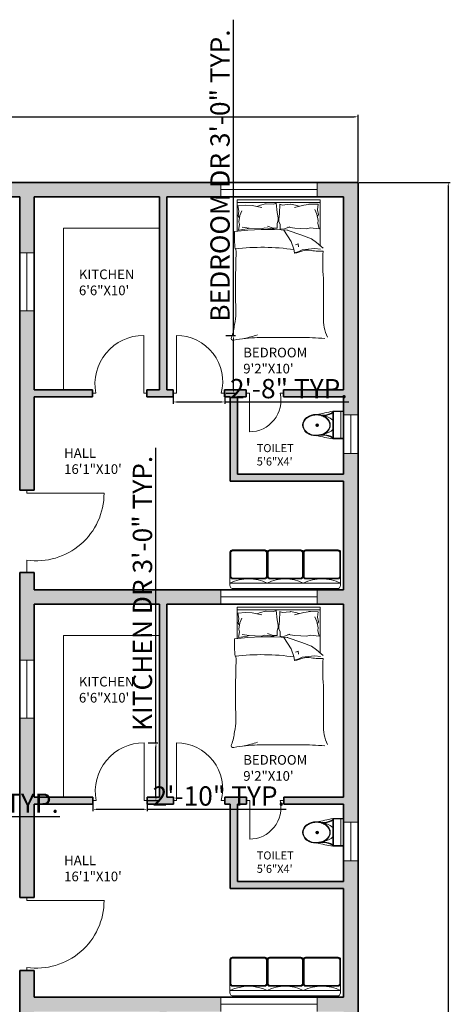
# Model space of a CAD drawing. Units: inches. Extents: x 1266 to 2869, y -408 to 3241.
# Tile 5 of 11: x 1748 to 2016, y 1767 to 2380. Entities that reach past the tile are written whole.
import ezdxf

# ---------------------------------------------------------------- set-up
doc = ezdxf.new("R2010")
doc.units = ezdxf.units.IN
for name, color, linetype, lineweight in [('A-ANNO-DIMS', 2, 'Continuous', 18), ('A-AREA-IDEN', 7, 'Continuous', 18), ('A-DOOR', 4, 'Continuous', 18), ('A-FLOR-CASE', 9, 'Continuous', 18), ('A-FLOR-FIXT', 9, 'Continuous', 18), ('A-FURN', 8, 'Continuous', 18), ('A-GLAZ', 4, 'Continuous', 18), ('A-WALL', 7, 'Continuous', 35), ('A-WALL-PATT', 251, 'Continuous', 13)]:
    doc.layers.add(name, color=color, linetype=linetype, lineweight=lineweight)
doc.styles.get("Standard").update_dxf_attribs({"font": 'arial.ttf'})
doc.dimstyles.new('ISO-25', dxfattribs={"dimtxt": 12, "dimasz": 2.5, "dimexe": 1.25, "dimexo": 0.625, "dimtad": 1, "dimdec": 0, "dimlunit": 3, "dimtxsty": 'Standard', "dimcen": 2.5, "dimadec": 0, "dimazin": 0, "dimtfac": 1, "dimtdec": 0, "dimtmove": 0, "dimatfit": 3, "dimfxl": 1, "dimarcsym": 0})

# ---------------------------------------------------------------- blocks, each defined once
blk = doc.blocks.new('A$C31115884')
for p, q in [((283, 498), (223, 498)), ((258, 466), (258, 523)), ((0, 200), (0, 0)), ((520, 200), (0, 200)), ((10, 190), (10, 10)), ((510, 190), (10, 190)), ((510, 10), (510, 190)), ((520, 0), (520, 200)), ((510, 54), (0, 54)), ((10, 10), (510, 10)), ((0, 0), (520, 0))]:
    blk.add_line(p, q)
blk.add_circle((256, 496), 23.6)
for centre, radius, start, end in [((2778, -205), 2807, 165.4549, 171.7133), ((-295, 403), 365, 324.2091, 9.3499), ((-295, 403), 375, 324.2091, 9.3499), ((139, 406), 293, 315.8436, 2.6563), ((806, 403), 375, 179.2036, 215.7909), ((806, 403), 365, 170.6501, 215.7909), ((3237, 905), 2807, 188.2867, 194.5451), ((384, 406), 293, 190.2774, 224.1564)]:
    blk.add_arc(centre, radius, start, end)
blk.add_ellipse((256, 510), major_axis=(0, -261), ratio=0.772727)
blk.add_open_spline([(256, 259), (263, 259), (270, 260), (288, 262), (299, 265), (320, 273), (330, 278), (350, 291), (360, 299), (378, 316), (386, 326), (402, 347), (409, 358), (421, 383), (427, 395), (436, 422), (440, 436), (445, 465), (447, 480), (448, 509), (448, 524), (445, 553), (443, 568), (436, 596), (432, 610), (422, 636), (416, 649), (402, 672), (395, 683), (379, 703), (370, 712), (351, 728), (341, 735), (321, 746), (310, 751), (289, 757), (278, 759), (256, 761), (245, 761), (223, 757), (212, 754), (191, 746), (181, 741), (161, 728), (151, 720), (133, 703), (125, 693), (110, 672), (103, 660), (90, 636), (85, 623), (76, 596), (72, 582), (67, 553), (66, 538), (64, 509), (65, 494), (68, 465), (70, 450), (77, 422), (81, 408), (91, 382), (97, 370), (111, 346), (118, 335), (135, 316), (144, 307), (162, 291), (172, 284), (193, 273), (203, 269), (225, 262), (236, 260), (250, 259), (253, 259), (256, 259)], degree=3, knots=[0, 0, 0, 0, 0.110105, 0.110105, 0.285049, 0.285049, 0.459994, 0.459994, 0.634938, 0.634938, 0.809882, 0.809882, 0.984827, 0.984827, 1.159771, 1.159771, 1.334715, 1.334715, 1.50966, 1.50966, 1.684604, 1.684604, 1.859549, 1.859549, 2.034493, 2.034493, 2.209437, 2.209437, 2.384382, 2.384382, 2.559326, 2.559326, 2.73427, 2.73427, 2.909215, 2.909215, 3.084159, 3.084159, 3.259103, 3.259103, 3.434048, 3.434048, 3.608992, 3.608992, 3.783936, 3.783936, 3.958881, 3.958881, 4.133825, 4.133825, 4.30877, 4.30877, 4.483714, 4.483714, 4.658658, 4.658658, 4.833603, 4.833603, 5.008547, 5.008547, 5.183491, 5.183491, 5.358436, 5.358436, 5.53338, 5.53338, 5.708324, 5.708324, 5.883269, 5.883269, 6.058213, 6.058213, 6.233158, 6.233158, 6.283185, 6.283185, 6.283185, 6.283185])
blk = doc.blocks.new('*D2')
at = {"layer": 'A-ANNO-DIMS', "color": 0, "lineweight": -2, "transparency": 16777216}
for p, q in [((1475.69, 2278.97), (1475.69, 2320.42)), ((1478.19, 2319.17), (1956.19, 2319.17)), ((1958.69, 2278.97), (1958.69, 2320.42))]:
    blk.add_line(p, q, dxfattribs=at)
at = {"layer": 'A-ANNO-DIMS', "color": 0, "transparency": 16777216}
for points in [[(1478.19, 2319.59), (1478.19, 2318.76), (1475.69, 2319.17)], [(1956.19, 2319.59), (1956.19, 2318.76), (1958.69, 2319.17)]]:
    blk.add_solid(points, dxfattribs=at)
at = {"layer": 'Defpoints', "color": 0, "transparency": 16777216}
for p in [(1958.69, 2319.17), (1475.69, 2278.35), (1958.69, 2278.35)]:
    blk.add_point(p, dxfattribs=at)
at = {"layer": 'A-ANNO-DIMS', "color": 0, "transparency": 16777216, "insert": (1717.19, 2325.93), "char_height": 12, "attachment_point": 5}
blk.add_mtext('40\'-3"', dxfattribs=at)
blk = doc.blocks.new('*D3')
at = {"layer": 'A-ANNO-DIMS', "color": 0, "lineweight": -2, "transparency": 16777216}
for p, q in [((1959.32, 2278.35), (2016.1, 2278.35)), ((2014.85, 2275.85), (2014.85, 1179.85)), ((1959.32, 1177.35), (2016.1, 1177.35))]:
    blk.add_line(p, q, dxfattribs=at)
at = {"layer": 'A-ANNO-DIMS', "color": 0, "transparency": 16777216}
for points in [[(2014.43, 2275.85), (2015.27, 2275.85), (2014.85, 2278.35)], [(2014.43, 1179.85), (2015.27, 1179.85), (2014.85, 1177.35)]]:
    blk.add_solid(points, dxfattribs=at)
at = {"layer": 'Defpoints', "color": 0, "transparency": 16777216}
for p in [(1958.69, 2278.35), (1958.69, 1177.35), (2014.85, 1177.35)]:
    blk.add_point(p, dxfattribs=at)
at = {"layer": 'A-ANNO-DIMS', "color": 0, "transparency": 16777216, "insert": (2008.1, 1727.85), "char_height": 12, "attachment_point": 5, "rotation": 90}
blk.add_mtext('91\'-9"', dxfattribs=at)
blk = doc.blocks.new('BED-DOUBLE-2')
for p, q in [((3.76, 67.77), (3.76, 87.35)), ((3.76, 87.35), (55.42, 87.35)), ((55.42, 87.35), (55.42, 58.59)), ((3.76, 85.69), (55.42, 85.69)), ((4.21, 83.74), (8.84, 84.1)), ((4.21, 83.77), (4.84, 80.33)), ((4.84, 80.33), (4.37, 77.51)), ((5.46, 77.67), (6.55, 80.64)), ((8.84, 84.1), (8.96, 84.08)), ((8.96, 84.08), (13.09, 83.77)), ((13.09, 83.77), (19.03, 82.67)), ((16.06, 83.3), (18.25, 84.08)), ((18.25, 84.08), (21.37, 84.86)), ((21.37, 84.86), (21.72, 84.86)), ((21.72, 84.86), (26.53, 84.7)), ((26.53, 84.7), (28.09, 85.33)), ((28.09, 85.33), (28.71, 79.55)), ((30.24, 84.66), (29.98, 78.85)), ((31.84, 84.13), (30.24, 84.66)), ((36.63, 84.59), (31.84, 84.13)), ((36.98, 84.61), (36.63, 84.59)), ((40.14, 84.02), (36.98, 84.61)), ((45.31, 84.03), (39.45, 82.57)), ((42.38, 83.38), (40.14, 84.02)), ((49.42, 84.6), (45.31, 84.03)), ((54.17, 84.59), (48.33, 84.69)), ((48.33, 84.69), (49.42, 84.6)), ((53.31, 78.43), (52.03, 81.32)), ((54.17, 84.59), (53.76, 81.12)), ((53.76, 81.12), (54.41, 78.34)), ((4.37, 77.51), (4.99, 76.42)), ((4.84, 73.76), (5.46, 77.67)), ((5.15, 72.04), (4.84, 73.76)), ((28.71, 79.55), (29.34, 76.11)), ((29.34, 74.7), (28.71, 72.67)), ((29.34, 76.11), (29.34, 74.7)), ((29.98, 78.85), (29.57, 75.38)), ((29.57, 75.38), (29.66, 73.97)), ((29.66, 73.97), (30.41, 71.98)), ((54.17, 74.56), (53.31, 78.43)), ((54.41, 78.34), (53.85, 77.21)), ((53.97, 72.83), (54.17, 74.56)), ((4.52, 68.61), (5.15, 72.04)), ((10.03, 69.39), (4.52, 68.61)), ((6.9, 70.46), (11.26, 69.74)), ((11.26, 69.74), (10.03, 69.39)), ((11.26, 69.74), (18.84, 69.27)), ((18.84, 69.27), (20.95, 69.87)), ((20.95, 69.87), (26.5, 69.44)), ((26.06, 69.77), (22.66, 70.95)), ((28.71, 69.77), (26.06, 69.77)), ((28.71, 72.67), (28.71, 69.77)), ((30.41, 71.98), (30.59, 69.09)), ((30.59, 69.09), (33.24, 69.26)), ((32.71, 68.56), (37.24, 61.54)), ((33.24, 69.26), (36.56, 70.64)), ((43.94, 65.39), (34.92, 68.56)), ((35.2, 70.46), (39.56, 69.74)), ((39.56, 69.74), (47.14, 69.27)), ((47.14, 69.27), (49.26, 69.87)), ((49.26, 69.87), (54.81, 69.44)), ((54.81, 69.44), (53.97, 72.83)), ((37.24, 61.54), (39.08, 56.69)), ((49.96, 63.21), (43.94, 65.39)), ((53.15, 60.87), (49.96, 63.21)), ((39.08, 56.69), (39.42, 54.51)), ((39.42, 54.51), (42.1, 55.18)), ((40.12, 59.32), (41.78, 59.99)), ((41.87, 58.1), (41.78, 59.99, 4.18)), ((42.1, 55.18), (44.27, 56.19)), ((44.27, 56.19), (47.96, 56.69)), ((47.96, 56.69), (52.14, 57.02)), ((52.14, 57.02), (55.49, 56.69)), ((57.15, 57.36), (53.15, 60.87)), ((16.28, 1.69), (42.89, 1.69))]:
    blk.add_line(p, q)
for centre, radius, start, end in [((92.06, 65.63), 90.06, 178.72178, 185.60397), ((23.09, -109.45), 178.34, 86.08655, 96.78213), ((19.19, -81.63), 139.47, 81.78449, 96.90062), ((-180.86, 53.65), 183.89, 358.4762, 1.00819), ((33.68, 85.75), 32.06, 280.66171, 289.88058), ((47.29, 49.44), 6.73, 78.6608, 113.73842), ((55.49, 94.55), 39.11, 259.87628, 272.56571), ((197.03, 48.09), 139.99, 176.97912, 183.83645), ((39.61, 54.45), 0.199, 160.24637, 271.13765), ((524.11, 32.64), 521.39, 178.22771, 181.71854), ((-4874.07, 14.03), 4931.49, 0.00217, 0.28689), ((-29.08, 17.61), 32.04, 346.06484, 358.91125), ((82.33, 13.12), 24.93, 177.47136, 206.46809), ((-23.41, 11.38), 25.47, 337.97508, 356.652), ((1.18, 1.17), 1.18, 146.17358, 293.47814), ((23.16, -129.76), 131.62, 92.99578, 99.40907), ((-18.62, 112.98), 115.08, 283.38322, 287.70533), ((44.49, -142.12), 143.82, 84.4998, 90.63509)]:
    blk.add_arc(centre, radius, start, end)
blk = doc.blocks.new('SOFA-3-SEAT-2')
for points in [[(0, 22.36), (0, 7.74, 0.414214), (1.72, 6.02), (21.5, 6.02, 0.414214), (23.22, 7.74), (23.22, 22.36, 0.414214), (21.5, 24.08), (1.72, 24.08, 0.414214)], [(0.52, 22.36), (0.52, 7.74, 0.414214), (1.72, 6.53), (21.5, 6.53, 0.414214), (22.7, 7.74), (22.7, 22.36, 0.414214), (21.5, 23.56), (1.72, 23.56, 0.414214)], [(45.57, 22.36), (45.57, 7.74, -0.414214), (43.85, 6.02), (24.94, 6.02, -0.414214), (23.22, 7.74), (23.22, 22.36, -0.414214), (24.94, 24.08), (43.85, 24.08, -0.414214)], [(45.06, 22.36), (45.06, 7.74, -0.414214), (43.85, 6.53), (24.94, 6.53, -0.414214), (23.73, 7.74), (23.73, 22.36, -0.414214), (24.94, 23.56), (43.85, 23.56, -0.414214)], [(45.57, 22.36), (45.57, 7.74, 0.414214), (47.29, 6.02), (67.07, 6.02, 0.414214), (68.79, 7.74), (68.79, 22.36, 0.414214), (67.07, 24.08), (47.29, 24.08, 0.414214)], [(46.09, 22.36), (46.09, 7.74, 0.414214), (47.29, 6.53), (67.07, 6.53, 0.414214), (68.27, 7.74), (68.27, 22.36, 0.414214), (67.07, 23.56), (47.29, 23.56, 0.414214)]]:
    blk.add_lwpolyline(points, format="xyb", close=True)
at = {"ltscale": 0.03}
blk.add_lwpolyline([(21.82, 24.08), (1.38, 24.08, 0.414214), (0, 22.7), (0, 2.06, 0.414214), (2.06, 0), (66.73, 0, 0.414214), (68.79, 2.06), (68.79, 22.7, 0.414214), (67.41, 24.08), (46.97, 24.08, 0.414214), (45.59, 22.7, -1), (45.56, 22.7, 0.414214), (44.18, 24.08), (24.61, 24.08, 0.414214), (23.23, 22.7, -1), (23.2, 22.7, 0.414214)], format="xyb", close=True, dxfattribs=at)
blk.add_lwpolyline([(0, 3.44), (68.79, 3.44)])
for centre, radius, start, end in [((11.61, -21.35), 27.38, 64.91063, 115.08937), ((34.4, -19.35), 25.38, 63.869, 116.131), ((57.18, -21.07), 27.12, 64.65382, 115.34618)]:
    blk.add_arc(centre, radius, start, end)
blk = doc.blocks.new('DOOR-KITCHEN-R')
for p, q in [((31.78, 0), (31.78, 36)), ((0, 0), (2, 0)), ((33.78, 0), (31.78, 0))]:
    blk.add_line(p, q)
blk.add_arc((31.78, 5.68), 30.32, 90, 190.7956)
blk = doc.blocks.new('DOOR-BEDROOM-R')
for p, q in [((2, 0), (2, 36)), ((0, 0), (2, 0)), ((31.84, 0), (29.84, 0))]:
    blk.add_line(p, q)
blk.add_arc((2, 7.24), 28.76, 345.43182, 90)
blk = doc.blocks.new('DOOR-BATH-R')
for p, q in [((0, 24), (2, 24)), ((2, 24), (2, 0)), ((23.14, 24), (21.14, 24))]:
    blk.add_line(p, q)
blk.add_arc((2, 19.63), 19.63, 270, 12.84994)
blk = doc.blocks.new('DOOR-ENTRY-R')
for p, q in [((0, 51.27), (0, 49.27)), ((0, 49.27), (36, 49.27)), ((36, 49.27), (48, 49.27)), ((0, 5.68), (0, 7.68)), ((0, 0), (0, 5.68))]:
    blk.add_line(p, q)
blk.add_arc((5.98, 49.27), 42.02, 261.81164, 0)
blk = doc.blocks.new('WIN-PLAN-60')
for p, q in [((0, 9), (0, 0)), ((60, 4.5), (60, 9)), ((60, 9), (60, 0)), ((0, 4.5), (60, 4.5)), ((0, 0), (0, 4.5))]:
    blk.add_line(p, q)
blk = doc.blocks.new('WIN-PLAN-36')
for p, q in [((0, 36), (9, 36)), ((4.5, 36), (4.5, 0)), ((9, 36), (4.5, 36)), ((4.5, 0), (0, 0)), ((0, 0), (9, 0))]:
    blk.add_line(p, q)
blk = doc.blocks.new('WIN-PLAN-24')
for p, q in [((0, 24), (9, 24)), ((4.5, 24), (4.5, 0)), ((9, 24), (4.5, 24)), ((0, 0), (9, 0))]:
    blk.add_line(p, q)
blk = doc.blocks.new('WIN-PLAN-24-2')
for p, q in [((0, 24), (9, 24)), ((4.5, 24), (4.5, 0)), ((9, 24), (4.5, 24)), ((4.5, 0), (0, 0)), ((0, 0), (9, 0))]:
    blk.add_line(p, q)
blk = doc.blocks.new('COUNTER-KITCHEN')
for p, q in [((0, 0), (0, 100.54)), ((0, 100.54), (59.82, 100.54))]:
    blk.add_line(p, q)
blk = doc.blocks.new('*D47')
at = {"layer": 'A-ANNO-DIMS', "color": 0, "lineweight": -2, "transparency": 16777216}
for p, q in [((1832.96, 1929.6), (1832.96, 2113.07)), ((1828.18, 1929.6), (1834.21, 1929.6)), ((1832.96, 1896.1), (1832.96, 1927.1)), ((1828.18, 1893.6), (1834.21, 1893.6))]:
    blk.add_line(p, q, dxfattribs=at)
at = {"layer": 'A-ANNO-DIMS', "color": 0, "transparency": 16777216}
for points in [[(1832.54, 1927.1), (1833.37, 1927.1), (1832.96, 1929.6)], [(1832.54, 1896.1), (1833.37, 1896.1), (1832.96, 1893.6)]]:
    blk.add_solid(points, dxfattribs=at)
at = {"layer": 'Defpoints', "color": 0, "transparency": 16777216}
for p in [(1827.56, 1929.6), (1832.96, 1929.6), (1827.56, 1893.6)]:
    blk.add_point(p, dxfattribs=at)
at = {"layer": 'A-ANNO-DIMS', "color": 0, "transparency": 16777216, "insert": (1826.12, 2022.58), "char_height": 12, "attachment_point": 5, "rotation": 90}
blk.add_mtext('KITCHEN DR 3\'-0" TYP.', dxfattribs=at)
blk = doc.blocks.new('*D48')
at = {"layer": 'A-ANNO-DIMS', "color": 0, "lineweight": -2, "transparency": 16777216}
for p, q in [((1793.77, 1892.97), (1793.77, 1886.95)), ((1796.27, 1888.2), (1825.06, 1888.2)), ((1827.56, 1892.97), (1827.56, 1886.95)), ((1827.56, 1888.2), (1913.98, 1888.2))]:
    blk.add_line(p, q, dxfattribs=at)
at = {"layer": 'A-ANNO-DIMS', "color": 0, "transparency": 16777216}
for points in [[(1796.27, 1888.61), (1796.27, 1887.78), (1793.77, 1888.2)], [(1825.06, 1888.61), (1825.06, 1887.78), (1827.56, 1888.2)]]:
    blk.add_solid(points, dxfattribs=at)
at = {"layer": 'Defpoints', "color": 0, "transparency": 16777216}
for p in [(1793.77, 1893.6), (1827.56, 1893.6), (1827.56, 1888.2)]:
    blk.add_point(p, dxfattribs=at)
at = {"layer": 'A-ANNO-DIMS', "color": 0, "transparency": 16777216, "insert": (1872.02, 1894.95), "char_height": 12, "attachment_point": 5}
blk.add_mtext('2\'-10" TYP.', dxfattribs=at)
blk = doc.blocks.new('*D55')
at = {"layer": 'A-ANNO-DIMS', "color": 0, "lineweight": -2, "transparency": 16777216}
for p, q in [((1881.22, 2183.1), (1881.22, 2379.61)), ((1876.44, 2183.1), (1882.47, 2183.1)), ((1881.22, 2149.6), (1881.22, 2180.6)), ((1876.44, 2147.1), (1882.47, 2147.1))]:
    blk.add_line(p, q, dxfattribs=at)
at = {"layer": 'A-ANNO-DIMS', "color": 0, "transparency": 16777216}
for points in [[(1880.8, 2180.6), (1881.63, 2180.6), (1881.22, 2183.1)], [(1880.8, 2149.6), (1881.63, 2149.6), (1881.22, 2147.1)]]:
    blk.add_solid(points, dxfattribs=at)
at = {"layer": 'Defpoints', "color": 0, "transparency": 16777216}
for p in [(1875.82, 2183.1), (1881.22, 2183.1), (1875.82, 2147.1)]:
    blk.add_point(p, dxfattribs=at)
at = {"layer": 'A-ANNO-DIMS', "color": 0, "transparency": 16777216, "insert": (1874.38, 2282.6), "char_height": 12, "attachment_point": 5, "rotation": 90}
blk.add_mtext('BEDROOM DR 3\'-0" TYP.', dxfattribs=at)
blk = doc.blocks.new('*D56')
at = {"layer": 'A-ANNO-DIMS', "color": 0, "lineweight": -2, "transparency": 16777216}
for p, q in [((1843.74, 2146.47), (1843.74, 2140.45)), ((1875.82, 2146.47), (1875.82, 2140.45)), ((1846.24, 2141.7), (1873.32, 2141.7)), ((1875.82, 2141.7), (1952.92, 2141.7))]:
    blk.add_line(p, q, dxfattribs=at)
at = {"layer": 'A-ANNO-DIMS', "color": 0, "transparency": 16777216}
for points in [[(1846.24, 2142.11), (1846.24, 2141.28), (1843.74, 2141.7)], [(1873.32, 2142.11), (1873.32, 2141.28), (1875.82, 2141.7)]]:
    blk.add_solid(points, dxfattribs=at)
at = {"layer": 'Defpoints', "color": 0, "transparency": 16777216}
for p in [(1843.74, 2147.1), (1875.82, 2147.1), (1875.82, 2141.7)]:
    blk.add_point(p, dxfattribs=at)
at = {"layer": 'A-ANNO-DIMS', "color": 0, "transparency": 16777216, "insert": (1915.62, 2148.45), "char_height": 12, "attachment_point": 5}
blk.add_mtext('2\'-8" TYP.', dxfattribs=at)
blk = doc.blocks.new('*D78')
at = {"layer": 'A-ANNO-DIMS', "color": 0, "lineweight": -2, "transparency": 16777216}
for p, q in [((1687.19, 1880.73), (1687.19, 1884.96)), ((1689.69, 1883.71), (1693.69, 1883.71)), ((1696.19, 1880.73), (1696.19, 1884.96)), ((1696.19, 1883.71), (1773.09, 1883.71))]:
    blk.add_line(p, q, dxfattribs=at)
at = {"layer": 'A-ANNO-DIMS', "color": 0, "transparency": 16777216}
for points in [[(1689.69, 1884.13), (1689.69, 1883.29), (1687.19, 1883.71)], [(1693.69, 1884.13), (1693.69, 1883.29), (1696.19, 1883.71)]]:
    blk.add_solid(points, dxfattribs=at)
at = {"layer": 'Defpoints', "color": 0, "transparency": 16777216}
for p in [(1696.19, 1883.71), (1687.19, 1880.11), (1696.19, 1880.11)]:
    blk.add_point(p, dxfattribs=at)
at = {"layer": 'A-ANNO-DIMS', "color": 0, "transparency": 16777216, "insert": (1735.89, 1890.46), "char_height": 12, "attachment_point": 5}
blk.add_mtext('0\'-9" TYP.', dxfattribs=at)

msp = doc.modelspace()

# ---------------------------------------------------------------- hatches: boundary and pattern name
at = {"layer": 'A-WALL-PATT'}
h = msp.add_hatch(color=256, dxfattribs=at)
h.dxf.hatch_style = 1
h.paths.add_polyline_path([(1484.69, 2269.35), (1562.69, 2269.35), (1562.69, 2149.35), (1558.42, 2149.35), (1558.42, 2144.85), (1567.19, 2144.85), (1573.23, 2144.85), (1573.23, 2146.74), (1573.23, 2149.35), (1567.19, 2149.35), (1567.19, 2269.35), (1597.45, 2269.35), (1597.45, 2273.85), (1597.45, 2278.35), (1475.69, 2278.35), (1475.69, 2234.52), (1484.69, 2234.52)])
h.paths.add_polyline_path([(1873.25, 2278.35), (1748.19, 2278.35), (1696.19, 2278.35), (1657.45, 2278.35), (1657.45, 2269.35), (1687.19, 2269.35), (1687.19, 2149.35), (1651.94, 2149.35), (1651.94, 2144.85), (1687.19, 2144.85), (1687.19, 2133.61), (1696.19, 2133.61), (1696.19, 2269.35), (1748.19, 2269.35), (1748.19, 2234.52), (1757.19, 2234.52), (1757.19, 2269.35), (1835.19, 2269.35), (1835.19, 2149.35), (1827.33, 2149.35), (1827.33, 2144.85), (1843.74, 2144.85), (1843.74, 2149.35), (1839.69, 2149.35), (1839.69, 2269.35), (1873.25, 2269.35), (1873.25, 2273.85)])
h.paths.add_polyline_path([(1958.69, 2278.35), (1933.25, 2278.35), (1933.25, 2269.35), (1949.69, 2269.35), (1949.69, 2149.35), (1912.22, 2149.35), (1912.22, 2144.85), (1949.69, 2144.85), (1949.69, 2133.61), (1958.69, 2133.61)])
h.paths.add_polyline_path([(1883.69, 2144.85), (1889.08, 2144.85), (1889.08, 2149.35), (1875.58, 2149.35), (1875.58, 2144.85), (1879.19, 2144.85), (1879.19, 2092.35), (1949.69, 2092.35), (1949.69, 2086.89), (1949.69, 2024.85), (1933.25, 2024.85), (1933.25, 2015.85), (1949.69, 2015.85), (1949.69, 1895.85), (1912.45, 1895.85), (1912.45, 1891.35), (1949.69, 1891.35), (1949.69, 1880.11), (1958.69, 1880.11), (1958.69, 2086.89), (1958.69, 2109.61), (1949.69, 2109.61), (1949.69, 2096.85), (1883.69, 2096.85)])
h.paths.add_polyline_path([(1757.19, 2198.52), (1748.19, 2198.52), (1748.19, 2086.89), (1757.19, 2086.89), (1757.19, 2144.85), (1793.55, 2144.85), (1793.55, 2149.35), (1757.19, 2149.35)])
h.paths.add_polyline_path([(1696.19, 2109.61), (1687.19, 2109.61), (1687.19, 2096.85), (1621.19, 2096.85), (1621.19, 2144.85), (1627.24, 2144.85), (1627.24, 2149.35), (1616.69, 2149.35), (1610.35, 2149.35), (1610.35, 2144.85), (1616.69, 2144.85), (1616.69, 2092.35), (1687.19, 2092.35), (1687.19, 2086.89), (1696.19, 2086.89)], flags=17)
h.paths.add_polyline_path([(1484.69, 2144.85), (1520.8, 2144.85), (1520.8, 2149.35), (1484.69, 2149.35), (1484.69, 2198.52), (1475.69, 2198.52), (1475.69, 1981.02), (1484.69, 1981.02), (1484.69, 2015.85), (1687.19, 2015.85), (1687.19, 1895.85), (1650.13, 1895.85), (1650.13, 1891.35), (1687.19, 1891.35), (1687.19, 1880.11), (1696.19, 1880.11), (1696.19, 2035.62), (1687.19, 2035.62), (1687.19, 2024.85), (1484.69, 2024.85)])
h.paths.add_polyline_path([(1484.69, 1691.52), (1475.69, 1691.52), (1475.69, 1474.02), (1484.69, 1474.02)])
h.paths.add_polyline_path([(1518.03, 1895.85), (1484.69, 1895.85), (1484.69, 1945.02), (1475.69, 1945.02), (1475.69, 1727.52), (1484.69, 1727.52), (1484.69, 1762.35), (1687.19, 1762.35), (1687.19, 1642.35), (1651.94, 1642.35), (1651.94, 1637.85), (1687.19, 1637.85), (1687.19, 1589.85), (1621.19, 1589.85), (1621.19, 1637.85), (1627.19, 1637.85), (1627.19, 1642.35), (1610.89, 1642.35), (1610.89, 1637.85), (1616.69, 1637.85), (1616.69, 1585.35), (1687.19, 1585.35), (1687.19, 1579.45), (1696.19, 1579.45), (1696.19, 1779.84), (1687.19, 1779.84), (1687.19, 1771.35), (1484.69, 1771.35), (1484.69, 1891.35), (1518.03, 1891.35)])
h.paths.add_polyline_path([(1567.19, 2015.85), (1562.69, 2015.85), (1562.69, 1895.85), (1555.64, 1895.85), (1555.64, 1891.35), (1570.46, 1891.35), (1570.46, 1895.85), (1567.19, 1895.85)], flags=17)
h.paths.add_polyline_path([(1625.43, 1895.85), (1607.58, 1895.85), (1607.58, 1891.35), (1616.69, 1891.35), (1616.69, 1838.85), (1687.19, 1838.85), (1687.19, 1831.11), (1696.19, 1831.11), (1696.19, 1856.11), (1687.19, 1856.11), (1687.19, 1843.35), (1621.19, 1843.35), (1621.19, 1891.35), (1625.43, 1891.35)], flags=17)
h.paths.add_polyline_path([(1567.19, 1762.35), (1562.69, 1762.35), (1562.69, 1642.35), (1558.42, 1642.35), (1558.42, 1637.85), (1573.23, 1637.85), (1573.23, 1642.35), (1567.19, 1642.35)], flags=17)
h.paths.add_polyline_path([(1520.8, 1642.35), (1484.69, 1642.35), (1484.69, 1637.85), (1520.8, 1637.85)], flags=17)
h.paths.add_polyline_path([(1687.19, 1517.85), (1484.69, 1517.85), (1484.69, 1508.85), (1562.69, 1508.85), (1562.69, 1388.85), (1567.19, 1388.85), (1567.19, 1508.85), (1687.19, 1508.85)])
h.paths.add_polyline_path([(1696.19, 1528.18), (1687.19, 1528.18), (1687.19, 1323.21), (1696.19, 1323.21)])
h.paths.add_polyline_path([(1696.19, 1271.94), (1687.19, 1271.94), (1687.19, 1264.35), (1484.69, 1264.35), (1484.69, 1283.77), (1480.19, 1283.77), (1475.69, 1283.77), (1475.69, 1255.35), (1480.19, 1255.35), (1696.19, 1255.35)])
h.paths.add_polyline_path([(1484.69, 1438.02), (1475.69, 1438.02), (1475.69, 1319.77), (1484.69, 1319.77)])
h.paths.add_polyline_path([(1873.25, 1513.35), (1873.25, 1517.85), (1757.19, 1517.85), (1757.19, 1528.62), (1748.19, 1528.62), (1748.19, 1474.02), (1757.19, 1474.02), (1757.19, 1508.85), (1835.19, 1508.85), (1835.19, 1388.85), (1827.33, 1388.85), (1827.33, 1384.35), (1843.74, 1384.35), (1843.74, 1388.85), (1839.69, 1388.85), (1839.69, 1508.85), (1873.25, 1508.85)])
h.paths.add_polyline_path([(1958.69, 1602.61), (1949.69, 1602.61), (1949.69, 1517.85), (1933.25, 1517.85), (1933.25, 1508.85), (1949.69, 1508.85), (1949.69, 1388.85), (1912.22, 1388.85), (1912.22, 1384.35), (1949.69, 1384.35), (1949.69, 1373.11), (1958.69, 1373.11)])
h.paths.add_polyline_path([(1958.69, 1349.11), (1949.69, 1349.11), (1949.69, 1336.35), (1883.69, 1336.35), (1883.69, 1384.35), (1889.08, 1384.35), (1889.08, 1388.85), (1875.58, 1388.85), (1875.58, 1384.35), (1879.19, 1384.35), (1879.19, 1331.85), (1949.69, 1331.85), (1949.69, 1315.59), (1958.69, 1315.59)])
h.paths.add_polyline_path([(1958.69, 1279.59), (1954.19, 1279.59), (1949.69, 1279.59), (1949.69, 1264.35), (1757.19, 1264.35), (1757.19, 1275.12), (1748.19, 1275.12), (1748.19, 1255.35), (1958.69, 1255.35)])
h.paths.add_polyline_path([(1757.19, 1438.02), (1748.19, 1438.02), (1748.19, 1326.39), (1757.19, 1326.39)])
h.paths.add_polyline_path([(1793.55, 1388.85), (1757.19, 1388.85), (1757.19, 1384.35), (1793.55, 1384.35)], flags=0)
h = msp.add_hatch(color=256, dxfattribs=at)
h.dxf.hatch_style = 1
h.paths.add_polyline_path([(1873.25, 2020.35), (1873.25, 2024.85), (1757.19, 2024.85), (1757.19, 2035.62), (1748.19, 2035.62), (1748.19, 1981.02), (1757.19, 1981.02), (1757.19, 2015.85), (1835.19, 2015.85), (1835.19, 1895.85), (1827.57, 1895.85), (1827.57, 1891.35), (1843.96, 1891.35), (1843.96, 1895.85), (1839.69, 1895.85), (1839.69, 2015.85), (1873.25, 2015.85)])
h.paths.add_polyline_path([(1757.19, 1945.02), (1748.19, 1945.02), (1748.19, 1833.39), (1757.19, 1833.39), (1757.19, 1891.35), (1793.77, 1891.35), (1793.77, 1895.85), (1757.19, 1895.85)])
h.paths.add_polyline_path([(1873.25, 1771.35), (1757.19, 1771.35), (1757.19, 1787.8), (1748.19, 1787.8), (1748.19, 1727.52), (1757.19, 1727.52), (1757.19, 1762.35), (1835.19, 1762.35), (1835.19, 1642.35), (1827.33, 1642.35), (1827.33, 1637.85), (1843.74, 1637.85), (1843.74, 1642.35), (1839.69, 1642.35), (1839.69, 1762.35), (1873.25, 1762.35), (1873.25, 1766.85)])
h.paths.add_polyline_path([(1883.69, 1637.85), (1889.08, 1637.85), (1889.08, 1642.35), (1875.58, 1642.35), (1875.58, 1637.85), (1879.19, 1637.85), (1879.19, 1585.35), (1949.69, 1585.35), (1949.69, 1589.85), (1883.69, 1589.85)])
h.paths.add_polyline_path([(1958.69, 1856.11), (1949.69, 1856.11), (1949.69, 1843.35), (1883.69, 1843.35), (1883.69, 1891.35), (1889.31, 1891.35), (1889.31, 1895.85), (1875.8, 1895.85), (1875.8, 1891.35), (1879.19, 1891.35), (1879.19, 1838.85), (1949.69, 1838.85), (1949.69, 1771.35), (1933.25, 1771.35), (1933.25, 1762.35), (1949.69, 1762.35), (1949.69, 1642.35), (1912.22, 1642.35), (1912.22, 1637.85), (1949.69, 1637.85), (1949.69, 1626.61), (1958.69, 1626.61)])
h.paths.add_polyline_path([(1757.19, 1691.52), (1748.19, 1691.52), (1748.19, 1579.89), (1757.19, 1579.89)])
h.paths.add_polyline_path([(1793.55, 1642.35), (1757.19, 1642.35), (1757.19, 1637.85), (1793.55, 1637.85)], flags=17)

# ---------------------------------------------------------------- linework, layer by layer
at = {"layer": 'A-DOOR'}
for p, q in [((1845.74, 1893.6), (1845.74, 1929.6)), ((1793.77, 1893.6), (1795.55, 1893.6)), ((1827.33, 1893.6), (1825.56, 1893.6)), ((1843.96, 1893.6), (1845.74, 1893.6)), ((1843.96, 1893.6), (1845.74, 1893.6)), ((1875.58, 1893.6), (1873.58, 1893.6)), ((1875.8, 1893.6), (1873.8, 1893.6)), ((1889.31, 1893.6), (1891.31, 1893.6)), ((1891.31, 1893.6), (1891.31, 1869.6)), ((1912.22, 1893.6), (1910.22, 1893.6)), ((1912.45, 1893.6), (1910.45, 1893.6)), ((1752.69, 1833.39), (1752.69, 1831.39)), ((1752.69, 1831.39), (1788.69, 1831.39)), ((1752.92, 1831.39), (1788.92, 1831.39)), ((1788.69, 1831.39), (1800.69, 1831.39)), ((1788.92, 1831.39), (1800.92, 1831.39)), ((1752.69, 1787.8), (1752.69, 1789.8))]:
    msp.add_line(p, q, dxfattribs=at)
for centre, radius, start, end in [((1845.74, 1900.83), 28.76, 345.43182, 90), ((1891.08, 1889.23), 19.63, 270, 12.84994), ((1758.68, 1831.39), 42.02, 261.81164, 0)]:
    msp.add_arc(centre, radius, start, end, dxfattribs=at)
at = {"layer": 'A-FURN'}
for points in [[(1879.02, 1794.38), (1879.02, 1779.76, 0.414214), (1880.74, 1778.04), (1900.51, 1778.04, 0.414214), (1902.23, 1779.76), (1902.23, 1794.38, 0.414214), (1900.51, 1796.1), (1880.74, 1796.1, 0.414214)], [(1879.53, 1794.38), (1879.53, 1779.76, 0.414214), (1880.74, 1778.56), (1900.51, 1778.56, 0.414214), (1901.72, 1779.76), (1901.72, 1794.38, 0.414214), (1900.51, 1795.59), (1880.74, 1795.59, 0.414214)], [(1924.59, 1794.38), (1924.59, 1779.76, -0.414214), (1922.87, 1778.04), (1903.95, 1778.04, -0.414214), (1902.23, 1779.76), (1902.23, 1794.38, -0.414214), (1903.95, 1796.1), (1922.87, 1796.1, -0.414214)], [(1924.07, 1794.38), (1924.07, 1779.76, -0.414214), (1922.87, 1778.56), (1903.95, 1778.56, -0.414214), (1902.75, 1779.76), (1902.75, 1794.38, -0.414214), (1903.95, 1795.59), (1922.87, 1795.59, -0.414214)], [(1924.59, 1794.38), (1924.59, 1779.76, 0.414214), (1926.31, 1778.04), (1946.09, 1778.04, 0.414214), (1947.81, 1779.76), (1947.81, 1794.38, 0.414214), (1946.09, 1796.1), (1926.31, 1796.1, 0.414214)], [(1925.11, 1794.38), (1925.11, 1779.76, 0.414214), (1926.31, 1778.56), (1946.09, 1778.56, 0.414214), (1947.29, 1779.76), (1947.29, 1794.38, 0.414214), (1946.09, 1795.59), (1926.31, 1795.59, 0.414214)]]:
    msp.add_lwpolyline(points, format="xyb", close=True, dxfattribs=at)
at = {"layer": 'A-FURN', "ltscale": 0.03}
msp.add_lwpolyline([(1900.84, 1796.1), (1880.39, 1796.1, 0.414214), (1879.02, 1794.73), (1879.02, 1774.09, 0.414214), (1881.08, 1772.03), (1945.74, 1772.03, 0.414214), (1947.81, 1774.09), (1947.81, 1794.73, 0.414214), (1946.43, 1796.1), (1925.98, 1796.1, 0.414214), (1924.61, 1794.73, -1), (1924.57, 1794.73, 0.414214), (1923.2, 1796.1), (1903.63, 1796.1, 0.414214), (1902.25, 1794.73, -1), (1902.22, 1794.73, 0.414214)], format="xyb", close=True, dxfattribs=at)
at = {"layer": 'A-FURN'}
msp.add_lwpolyline([(1879.02, 1775.47), (1947.81, 1775.47)], dxfattribs=at)
for centre, radius, start, end in [((1890.62, 1750.67), 27.38, 64.91063, 115.08937), ((1913.41, 1752.68), 25.38, 63.869, 116.131), ((1936.2, 1750.96), 27.12, 64.65382, 115.34618)]:
    msp.add_arc(centre, radius, start, end, dxfattribs=at)
at = {"layer": 'A-WALL'}
for p, q in [((1696.19, 2278.35), (1748.19, 2278.35)), ((1748.19, 2278.35), (1958.69, 2278.35)), ((1958.69, 2278.35), (1958.69, 2086.89)), ((1748.19, 2269.35), (1696.19, 2269.35)), ((1748.19, 2269.35), (1748.19, 2086.89)), ((1757.19, 2269.35), (1757.19, 2149.35)), ((1757.19, 2269.35), (1835.19, 2269.35)), ((1835.19, 2269.35), (1835.19, 2149.35)), ((1839.69, 2269.35), (1839.69, 2149.35)), ((1839.69, 2269.35), (1949.69, 2269.35)), ((1949.69, 2269.35), (1949.69, 2149.35)), ((1757.19, 2149.35), (1793.55, 2149.35)), ((1757.19, 2144.85), (1793.55, 2144.85)), ((1757.19, 2144.85), (1757.19, 2086.89)), ((1793.55, 2149.35), (1793.55, 2144.85)), ((1827.33, 2149.35), (1827.33, 2144.85)), ((1827.33, 2149.35), (1835.19, 2149.35)), ((1827.33, 2144.85), (1843.74, 2144.85)), ((1839.69, 2149.35), (1843.74, 2149.35)), ((1843.74, 2149.35), (1843.74, 2144.85)), ((1843.74, 2149.35), (1843.74, 2144.85)), ((1875.58, 2149.35), (1875.58, 2144.85)), ((1875.58, 2149.35), (1889.08, 2149.35)), ((1875.58, 2144.85), (1879.19, 2144.85)), ((1879.19, 2144.85), (1879.19, 2092.35)), ((1883.69, 2144.85), (1883.69, 2096.85)), ((1883.69, 2144.85), (1889.08, 2144.85)), ((1889.08, 2149.35), (1889.08, 2144.85)), ((1912.22, 2149.35), (1912.22, 2144.85)), ((1912.22, 2149.35), (1949.69, 2149.35)), ((1912.22, 2144.85), (1949.69, 2144.85)), ((1949.69, 2144.85), (1949.69, 2096.85)), ((1883.69, 2096.85), (1949.69, 2096.85)), ((1879.19, 2092.35), (1949.69, 2092.35)), ((1949.69, 2092.35), (1949.69, 2086.89)), ((1748.19, 2086.89), (1757.19, 2086.89)), ((1949.69, 2086.89), (1949.69, 2024.85)), ((1958.69, 1255.35), (1958.69, 2086.89)), ((1748.19, 2035.62), (1748.19, 1833.39)), ((1748.19, 2035.62), (1757.19, 2035.62)), ((1757.19, 2035.62), (1757.19, 2024.85)), ((1757.19, 2024.85), (1949.69, 2024.85)), ((1757.19, 2015.85), (1835.19, 2015.85)), ((1757.19, 2015.85), (1757.19, 1895.85)), ((1835.19, 2015.85), (1835.19, 1895.85)), ((1839.69, 2015.85), (1839.69, 1895.85)), ((1839.69, 2015.85), (1949.69, 2015.85)), ((1949.69, 2015.85), (1949.69, 1895.85)), ((1757.19, 1895.85), (1793.77, 1895.85)), ((1793.77, 1893.6), (1793.77, 1895.85)), ((1793.77, 1895.85), (1793.77, 1891.35)), ((1827.57, 1891.35), (1827.57, 1895.85)), ((1827.57, 1895.85), (1835.19, 1895.85)), ((1839.69, 1895.85), (1843.96, 1895.85)), ((1843.96, 1891.35), (1843.96, 1895.85)), ((1843.96, 1893.6), (1843.96, 1891.35)), ((1875.8, 1891.35), (1875.8, 1895.85)), ((1875.8, 1895.85), (1889.31, 1895.85)), ((1875.8, 1893.6), (1875.8, 1891.35)), ((1889.31, 1891.35), (1889.31, 1895.85)), ((1912.45, 1891.35), (1912.45, 1895.85)), ((1912.45, 1895.85), (1949.69, 1895.85)), ((1912.45, 1893.6), (1912.45, 1891.35)), ((1757.19, 1891.35), (1793.77, 1891.35)), ((1757.19, 1891.35), (1757.19, 1833.39)), ((1827.57, 1891.35), (1843.96, 1891.35)), ((1875.8, 1891.35), (1879.19, 1891.35)), ((1879.19, 1891.35), (1879.19, 1838.85)), ((1883.69, 1891.35), (1883.69, 1843.35)), ((1883.69, 1891.35), (1889.31, 1891.35)), ((1912.45, 1891.35), (1912.45, 1891.35)), ((1912.45, 1891.35), (1949.69, 1891.35)), ((1949.69, 1891.35), (1949.69, 1843.35)), ((1879.19, 1838.85), (1949.69, 1838.85)), ((1883.69, 1843.35), (1949.69, 1843.35)), ((1949.69, 1838.85), (1949.69, 1771.35)), ((1752.92, 1833.39), (1748.19, 1833.39)), ((1748.19, 1833.39), (1757.19, 1833.39)), ((1757.19, 1787.8), (1748.19, 1787.8)), ((1748.19, 1787.8), (1748.19, 1579.89)), ((1752.92, 1787.8), (1757.19, 1787.8)), ((1757.19, 1787.8), (1757.19, 1771.35)), ((1757.19, 1771.35), (1949.69, 1771.35))]:
    msp.add_line(p, q, dxfattribs=at)

# ---------------------------------------------------------------- block references
at = {"layer": 'A-DOOR'}
for name, p in [('DOOR-KITCHEN-R', (1793.55, 2147.1)), ('DOOR-BEDROOM-R', (1843.73, 2147.1)), ('DOOR-BATH-R', (1889.08, 2123.1)), ('DOOR-ENTRY-R', (1752.69, 2035.62)), ('DOOR-KITCHEN-R', (1793.77, 1893.6))]:
    msp.add_blockref(name, p, dxfattribs=at)
at = {"layer": 'A-FLOR-CASE'}
for p in [(1775.37, 2149.35), (1775.37, 1895.85)]:
    msp.add_blockref('COUNTER-KITCHEN', p, dxfattribs=at)
at = {"layer": 'A-FLOR-FIXT', "xscale": 0.0330640103915726, "yscale": 0.0330640103915726, "zscale": 0.0330640103915726, "rotation": 89.99999999999996}
for p in [(1949.69, 2118.81), (1949.69, 1865.31)]:
    msp.add_blockref('A$C31115884', p, dxfattribs=at)
at = {"layer": 'A-FURN'}
for name, p in [('BED-DOUBLE-2', (1879.75, 2180.11)), ('SOFA-3-SEAT-2', (1879.02, 2025.53)), ('BED-DOUBLE-2', (1879.75, 1926.61))]:
    msp.add_blockref(name, p, dxfattribs=at)
at = {"layer": 'A-GLAZ'}
for name, p in [('WIN-PLAN-60', (1873.25, 2269.35)), ('WIN-PLAN-36', (1748.19, 2198.52)), ('WIN-PLAN-24-2', (1949.69, 2109.61)), ('WIN-PLAN-60', (1873.25, 2015.85)), ('WIN-PLAN-36', (1748.19, 1945.02)), ('WIN-PLAN-24', (1949.69, 1856.11)), ('WIN-PLAN-60', (1873.25, 1762.35))]:
    msp.add_blockref(name, p, dxfattribs=at)

# ---------------------------------------------------------------- texts
at = {"layer": 'A-AREA-IDEN', "attachment_point": 1}
for s, width, insert, char_height in [('KITCHEN\\P6\'6"X10\'', 112.1355, (1785.05, 2224.14), 6), ('BEDROOM\\P9\'2"X10\'', 62.026, (1887.3, 2175.46), 6), ('TOILET\\P5\'6"X4\'', 46.3569, (1895.7, 2115.49), 5), ('HALL\\P16\'1"X10\'', 100.9767, (1775.86, 2112.93), 6), ('KITCHEN\\P6\'6"X10\'', 112.1355, (1785.05, 1970.64), 6), ('BEDROOM\\P9\'2"X10\'', 62.026, (1887.3, 1921.96), 6), ('HALL\\P16\'1"X10\'', 100.9767, (1775.86, 1859.43), 6), ('TOILET\\P5\'6"X4\'', 46.3569, (1895.7, 1861.99), 5)]:
    msp.add_mtext_dynamic_manual_height_columns(s, width=width, gutter_width=12.5, heights=[0], dxfattribs=dict(at, insert=insert, char_height=char_height))

# ---------------------------------------------------------------- dimensions: what is measured, and where the dimension line sits
at = {"layer": 'A-ANNO-DIMS'}
for base, p1, p2, text, picture, middle in [((1881.22, 2183.1), (1875.82, 2147.1), (1875.82, 2183.1), 'BEDROOM DR <> TYP.', '*D55', (1874.38, 2282.6)), ((1832.96, 1929.6), (1827.56, 1893.6), (1827.56, 1929.6), 'KITCHEN DR <> TYP.', '*D47', (1826.12, 2022.58))]:
    dim = msp.add_linear_dim(base=base, p1=p1, p2=p2, angle=90, text=text, dimstyle='ISO-25', override={"dimdec": 1, "dimlfac": 1, "dimrnd": 0, "dimzin": 1, "dimdsep": 46, "dimlunit": 4, "dimfrac": 2}, dxfattribs=at)
    dim.commit()
    dim.dimension.update_dxf_attribs({"geometry": picture, "text_midpoint": middle})
dim = msp.add_linear_dim(base=(1958.69, 2319.17), p1=(1475.69, 2278.35), p2=(1958.69, 2278.35), dimstyle='ISO-25', override={"dimclrd": 0, "dimclre": 0, "dimclrt": 0}, dxfattribs=at)
dim.commit()
dim.dimension.update_dxf_attribs({"geometry": '*D2', "text_midpoint": (1717.19, 2319.17), "dimtype": 160})
dim = msp.add_linear_dim(base=(2014.85, 1177.35), p1=(1958.69, 2278.35), p2=(1958.69, 1177.35), angle=90, dimstyle='ISO-25', override={"dimclrd": 0, "dimclre": 0, "dimclrt": 0}, dxfattribs=at)
dim.commit()
dim.dimension.update_dxf_attribs({"geometry": '*D3', "text_midpoint": (2008.1, 1727.85)})
for base, p1, p2, picture, middle in [((1875.82, 2141.7), (1843.74, 2147.1), (1875.82, 2147.1), '*D56', (1915.62, 2148.45)), ((1827.56, 1888.2), (1793.77, 1893.6), (1827.56, 1893.6), '*D48', (1872.02, 1894.95)), ((1696.19, 1883.71), (1687.19, 1880.11), (1696.19, 1880.11), '*D78', (1735.89, 1890.46))]:
    dim = msp.add_linear_dim(base=base, p1=p1, p2=p2, text='<> TYP.', dimstyle='ISO-25', override={"dimdec": 1, "dimlfac": 1, "dimrnd": 0, "dimzin": 1, "dimdsep": 46, "dimlunit": 4, "dimfrac": 2}, dxfattribs=at)
    dim.commit()
    dim.dimension.update_dxf_attribs({"geometry": picture, "text_midpoint": middle})

doc.saveas('drawing.dxf')
